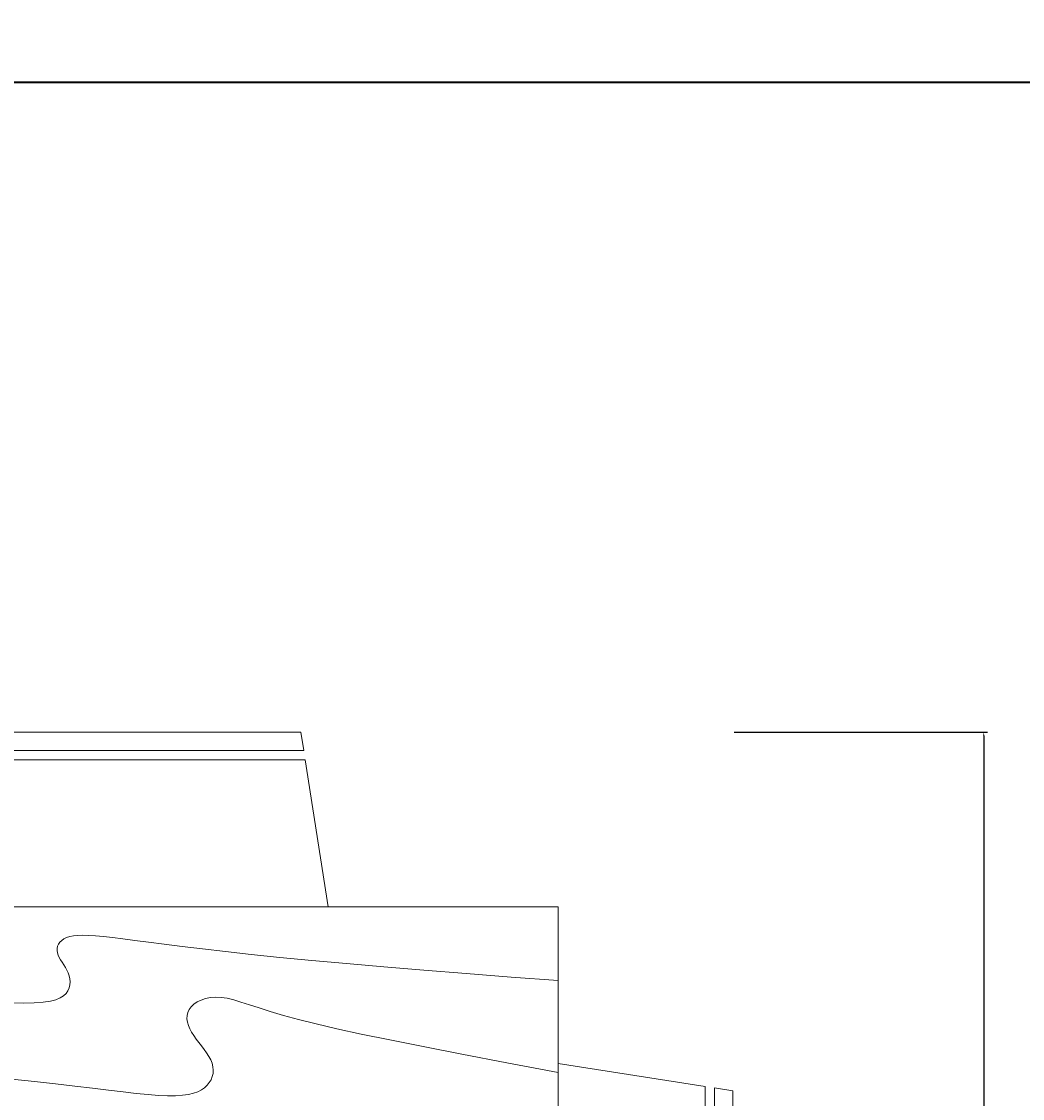
# Model space of a CAD drawing. Units: inches. Extents: x 4159 to 4826, y 299 to 1026.
# Tile 25 of 37: x 4354 to 4402, y 611 to 663. Entities that reach past the tile are written whole.
import ezdxf

# ---------------------------------------------------------------- set-up
doc = ezdxf.new("R2010")
doc.units = ezdxf.units.IN
for name, color, linetype, lineweight in [('A-ANNO-DIMS', 2, 'Continuous', 18), ('A-FURN', 8, 'Continuous', 18), ('A-WALL', 7, 'Continuous', 35)]:
    doc.layers.add(name, color=color, linetype=linetype, lineweight=lineweight)
doc.styles.get("Standard").update_dxf_attribs({"font": 'arial.ttf'})
doc.dimstyles.get("Standard").update_dxf_attribs({"dimtxt": 0.18, "dimasz": 0.18, "dimexe": 0.18, "dimexo": 0.0625, "dimgap": 0.09, "dimtad": 0, "dimtih": 1, "dimtoh": 1, "dimdec": 4, "dimzin": 0, "dimdsep": 46, "dimtxsty": 'Standard', "dimcen": 0.09, "dimadec": 0, "dimazin": 0, "dimtfac": 1, "dimtdec": 4, "dimtofl": 0, "dimtmove": 0, "dimatfit": 3, "dimfxl": 1, "dimtolj": 1, "dimtzin": 0, "dimarcsym": 0})

# ---------------------------------------------------------------- blocks, each defined once
blk = doc.blocks.new('Dining Set - 36 x 72 in.')
for p, q in [((6, 27.5), (22, 27.5)), ((22.1563, 26.49966), (22, 27.5)), ((22.1584, 26.5), (5.8466, 26.5)), ((5.7696, 26), (22.2392, 26)), ((23.4848, 17.99762), (22.2345, 25.99926)), ((36, 18), (-36, 18)), ((36, -18), (36, 18)), ((44.0006, 8.23428), (35.9976, 9.48474)), ((44, 8.23041), (44, -8.23915)), ((44.5, -8.15843), (44.5, 8.15338)), ((45.5, 8), (44.5005, 8.15617)), ((45.5, 8), (45.5, -8))]:
    blk.add_line(p, q)
for points in [[(6.1393, 12.78613), (6.8802, 12.76823), (7.4883, 12.77767), (7.9792, 12.8125), (8.3685, 12.87077), (8.6719, 12.95052), (8.9049, 13.0498), (9.0833, 13.16666), (9.2205, 13.29899), (9.3216, 13.44401), (9.3895, 13.59879), (9.4271, 13.76041), (9.4373, 13.92594), (9.4232, 14.09245), (9.3875, 14.257), (9.3333, 14.41666), (9.2638, 14.56917), (9.1836, 14.71484), (9.0975, 14.85465), (9.0104, 14.98958), (8.9272, 15.1206), (8.8529, 15.2487), (8.7922, 15.37483), (8.75, 15.5), (8.7305, 15.62467), (8.7344, 15.74739), (8.7617, 15.86621), (8.8125, 15.97916), (8.8867, 16.08431), (8.9844, 16.17968), (9.1055, 16.26334), (9.25, 16.33333), (9.4189, 16.38802), (9.6172, 16.42708), (9.8506, 16.45052), (10.125, 16.45833), (10.4463, 16.45052), (10.8203, 16.42708), (11.2529, 16.38802), (11.75, 16.33333), (12.3184, 16.26318), (12.9694, 16.17838), (13.7151, 16.07991), (14.5677, 15.96875), (15.5395, 15.84586), (16.6426, 15.71224), (17.8893, 15.56884), (19.2917, 15.41666), (20.859, 15.25667), (22.5879, 15.08984), (24.4721, 14.91715), (26.5052, 14.73958), (28.6809, 14.5581), (30.9929, 14.3737), (33.4347, 14.18733), (36, 14)], [(6.266, 8.62516), (7.5, 8.5), (8.6411, 8.37549), (9.6914, 8.2539), (10.6538, 8.13818), (11.5312, 8.03125), (12.3267, 7.93603), (13.043, 7.85547), (13.6831, 7.79248), (14.25, 7.75), (14.7471, 7.7303), (15.1797, 7.73307), (15.5537, 7.75732), (15.875, 7.80208), (16.1494, 7.86637), (16.3828, 7.94922), (16.5811, 8.04964), (16.75, 8.16666), (16.8944, 8.29915), (17.0143, 8.44531), (17.1089, 8.60319), (17.1771, 8.77083), (17.218, 8.94629), (17.2305, 9.1276), (17.2137, 9.31282), (17.1667, 9.5), (17.0895, 9.6875), (16.987, 9.875), (16.8649, 10.0625), (16.7292, 10.25), (16.5856, 10.4375), (16.4401, 10.625), (16.2985, 10.8125), (16.1667, 11), (16.05, 11.18733), (15.9518, 11.3737), (15.8752, 11.5581), (15.8229, 11.73958), (15.798, 11.91715), (15.8034, 12.08984), (15.842, 12.25667), (15.9167, 12.41666), (16.0295, 12.56836), (16.1784, 12.70833), (16.3605, 12.83268), (16.5729, 12.9375), (16.8127, 13.01888), (17.0768, 13.07291), (17.3625, 13.0957), (17.6667, 13.08333), (17.9894, 13.03312), (18.3418, 12.94726), (18.7382, 12.82918), (19.1927, 12.68229), (19.7195, 12.51001), (20.3327, 12.31575), (21.0465, 12.10294), (21.875, 11.875), (22.8357, 11.63354), (23.959, 11.37304), (25.2786, 11.08618), (26.8282, 10.76562), (28.6414, 10.40405), (30.752, 9.99414), (33.1936, 9.52856), (36, 9)]]:
    blk.add_lwpolyline(points)
blk = doc.blocks.new('*D36')
at = {"layer": 'A-ANNO-DIMS', "color": 0, "lineweight": -2, "transparency": 16777216}
for p, q in [((4388.337, 628.759), (4400.621, 628.759)), ((4400.441, 628.579), (4400.441, 604.428)), ((4400.441, 579.914), (4400.441, 604.064)), ((4388.337, 579.734), (4400.621, 579.734))]:
    blk.add_line(p, q, dxfattribs=at)
at = {"layer": 'A-ANNO-DIMS', "color": 0, "transparency": 16777216}
for points in [[(4400.411, 628.579), (4400.471, 628.579), (4400.441, 628.759)], [(4400.411, 579.914), (4400.471, 579.914), (4400.441, 579.734)]]:
    blk.add_solid(points, dxfattribs=at)
at = {"layer": 'Defpoints', "color": 0, "transparency": 16777216}
for p in [(4388.274, 628.759), (4400.441, 628.759), (4388.274, 579.734)]:
    blk.add_point(p, dxfattribs=at)
at = {"layer": 'A-ANNO-DIMS', "color": 0, "transparency": 16777216, "insert": (4400.441, 604.246), "char_height": 0.18, "attachment_point": 5}
blk.add_mtext('\\A1;49 TYP.', dxfattribs=at)
blk = doc.blocks.new('*D44')
at = {"layer": 'A-ANNO-DIMS', "color": 0, "lineweight": -2, "transparency": 16777216}
for p, q in [((4287.263, 963.093), (4158.88, 963.093)), ((4159.06, 962.913), (4159.06, 647.826)), ((4159.06, 332.375), (4159.06, 647.462)), ((4447.248, 332.195), (4158.88, 332.195))]:
    blk.add_line(p, q, dxfattribs=at)
at = {"layer": 'A-ANNO-DIMS', "color": 0, "transparency": 16777216}
for points in [[(4159.03, 962.913), (4159.09, 962.913), (4159.06, 963.093)], [(4159.03, 332.375), (4159.09, 332.375), (4159.06, 332.195)]]:
    blk.add_solid(points, dxfattribs=at)
at = {"layer": 'Defpoints', "color": 0, "transparency": 16777216}
for p in [(4287.326, 963.093), (4159.06, 332.195), (4447.31, 332.195)]:
    blk.add_point(p, dxfattribs=at)
at = {"layer": 'A-ANNO-DIMS', "color": 0, "transparency": 16777216, "insert": (4159.06, 647.644), "char_height": 0.18, "attachment_point": 5}
blk.add_mtext('\\A1;630.9', dxfattribs=at)

msp = doc.modelspace()

# ---------------------------------------------------------------- linework, layer by layer
at = {"layer": 'A-WALL'}
msp.add_line((4447.31, 660.254), (4201.31, 660.254), dxfattribs=at)

# ---------------------------------------------------------------- block references
at = {"layer": 'A-FURN', "xscale": 0.8913588978043845, "yscale": 0.8913588978043845, "zscale": 0.8913588978043845}
msp.add_blockref('Dining Set - 36 x 72 in.', (4347.717, 604.246), dxfattribs=at)

# ---------------------------------------------------------------- dimensions: what is measured, and where the dimension line sits
at = {"layer": 'A-ANNO-DIMS'}
dim = msp.add_linear_dim(base=(4159.06, 332.195), p1=(4287.326, 963.093), p2=(4447.31, 332.195), angle=90, dimstyle='Standard', override={"dimdec": 1, "dimlfac": 1, "dimrnd": 0, "dimzin": 0, "dimdsep": 46, "dimlunit": 2}, dxfattribs=at)
dim.commit()
dim.dimension.update_dxf_attribs({"geometry": '*D44', "text_midpoint": (4159.06, 647.644)})
dim = msp.add_linear_dim(base=(4400.441, 628.759), p1=(4388.274, 579.734), p2=(4388.274, 628.759), angle=90, text='<> TYP.', dimstyle='Standard', override={"dimdec": 0, "dimlfac": 1, "dimrnd": 0, "dimzin": 0, "dimdsep": 46, "dimlunit": 2}, dxfattribs=at)
dim.commit()
dim.dimension.update_dxf_attribs({"geometry": '*D36', "text_midpoint": (4400.441, 604.246)})

doc.saveas('drawing.dxf')
